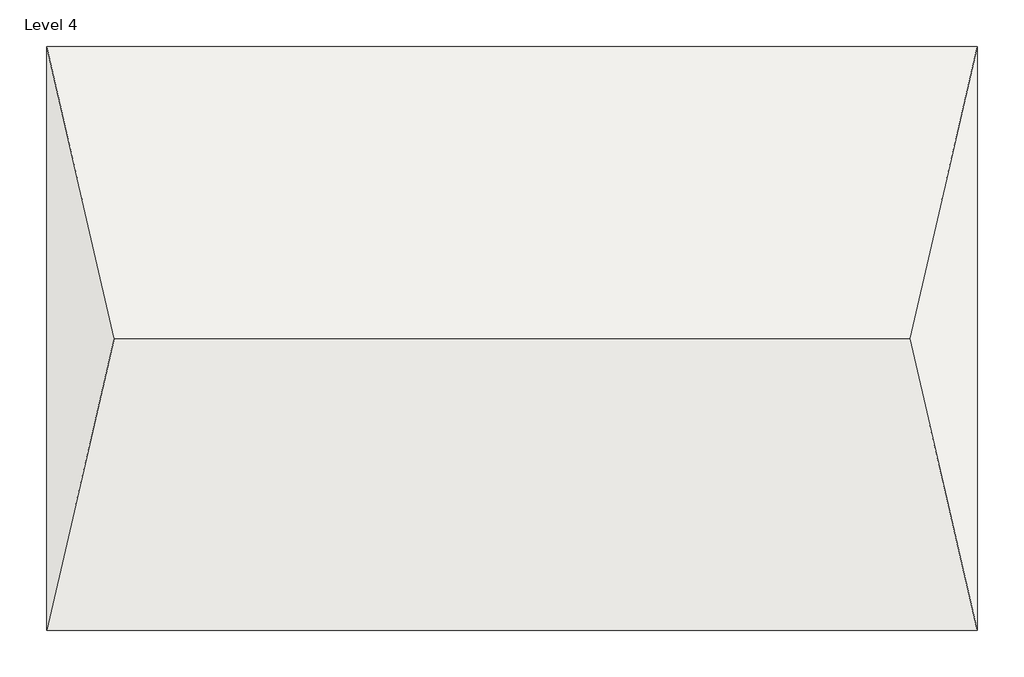
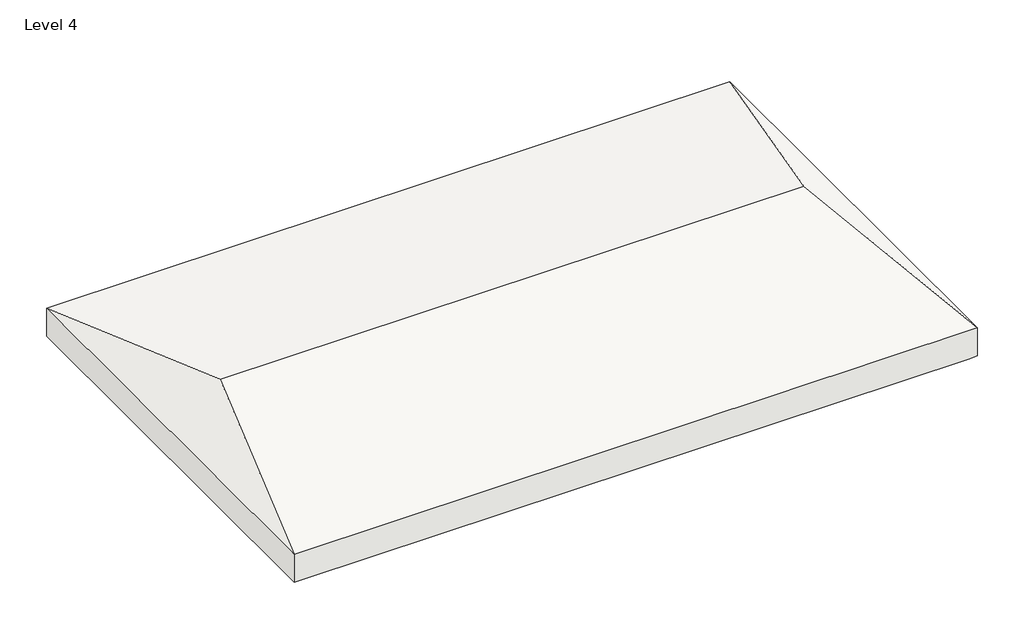
# One storey: 1 roof.
"""IFC4 building model written with IfcOpenShell, lengths in millimetres."""

from ifc_helpers import new_model, si_unit, origin, place, context, project, spatial, faceted_brep, element, save

model = new_model("IFC4")

# Units and contexts
model_context = context("Model", 3, world=origin())
ifc_project = project(units=[si_unit("LENGTHUNIT", "METRE", prefix="MILLI")], contexts=[model_context])

# Site, building, storey
site = spatial("IfcSite", under=ifc_project)
building = spatial("IfcBuilding", under=site)
storey = spatial("IfcBuildingStorey", under=building, Name="Level 4", Elevation=8839.2)

# Roof
placement = place(None, origin())
element("IfcRoof", 1, ObjectType="6\"", at=placement, inside=storey, context=model_context, shape_type="Brep", body=[
    faceted_brep([(-4209.088814, 1513.6825188, 8839.2), (-4468.3091453, 399.5187312, 9033.6152484), (-7406.514718, 399.5187312, 9033.6152484), (-7665.7350493, 1513.6825188, 8839.2), (-7665.7350493, -714.6450563, 8839.2), (-4209.088814, -714.6450563, 8839.2), (-4161.3591614, 1513.6825188, 8993.9027606), (-7713.4647018, 1513.6825188, 8993.9027606), (-7454.2443706, 399.5187312, 9188.318009), (-4420.5794927, 399.5187312, 9188.318009), (-7713.4647018, -714.6450563, 8993.9027606), (-4161.3591614, -714.6450563, 8993.9027606), (-7713.4647018, 1513.6825188, 8839.2), (-4161.3591614, 1513.6825188, 8839.2), (-7713.4647018, -714.6450563, 8839.2), (-4161.3591614, -714.6450563, 8839.2)], [[[0, 1, 2, 3]], [[3, 2, 4]], [[4, 2, 1, 5]], [[1, 0, 5]], [[6, 7, 8, 9]], [[7, 10, 8]], [[10, 11, 9, 8]], [[6, 9, 11]], [[12, 7, 6, 13, 0, 3]], [[14, 10, 7, 12]], [[15, 11, 10, 14, 4, 5]], [[13, 6, 11, 15]], [[13, 15, 5, 0]], [[4, 14, 12, 3]]]),
])

save(model, "model.ifc")

# Revit data of these elements
# Type "6\""
#   Assembly Code = "B1020"
#   Layers, outside or top first: 0' - 6" no material (function 1)
# Element 1 (IfcRoof, "6\"")
#   built-in parameter 1001705 = 30.1454 (stored number, unit not read)
#   built-in parameter 1001710 = 33615
#   Phase Created = New Construction
#   Materials on its faces: "Default Roof"
# Materials
#   "Default Roof": colour RGB 88 101 114, transparency 0
